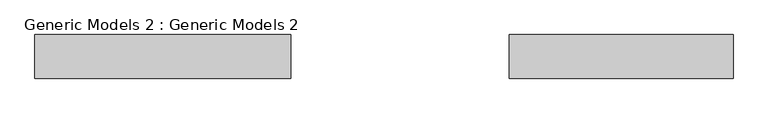
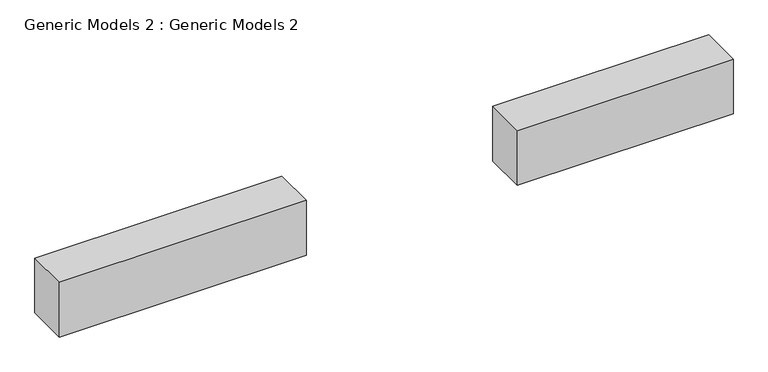
"""IFC4 building model written with IfcOpenShell, lengths in millimetres: proxy geometry, Generic Models 2 : Generic Models 2."""

from ifc_helpers import new_model, si_unit, frame, origin, place, context, project, spatial, polyline, outline, extrude, source, transform, mapped, element, save


def generic_models_2_generic_models_2_263b720d(model_context):
    return source(origin(), model_context, "Body", "SweptSolid", [
        extrude(outline(polyline([(-3264.7966546, -3075.5600272), (-5051.4108866, -3075.5600272), (-5051.4108866, -2770.7600272), (-3264.7966546, -2770.7600272), (-3264.7966546, -3075.5600272)])), frame((0.0, 0.0, 2476.1418569), z_axis=(0.0, 0.0, 1.0), x_axis=(1.0, 0.0, 0.0)), (0.0, 0.0, 1.0), 419.4581431),
        extrude(outline(polyline([(-174.6108866, -3075.5600272), (-1736.7108866, -3075.5600272), (-1736.7108866, -2770.7600272), (-174.6108866, -2770.7600272), (-174.6108866, -3075.5600272)])), frame((0.0, 0.0, 2476.1418569), z_axis=(0.0, 0.0, 1.0), x_axis=(1.0, 0.0, 0.0)), (0.0, 0.0, 1.0), 419.4581431),
    ])


if __name__ == "__main__":
    model = new_model("IFC4")
    model_context = context("Model", 3, world=origin())
    ifc_project = project(units=[si_unit("LENGTHUNIT", "METRE", prefix="MILLI")], contexts=[model_context])
    site = spatial("IfcSite", under=ifc_project)
    building = spatial("IfcBuilding", under=site)
    placement = place(None, origin())
    generic_models_2_generic_models_2_shape = generic_models_2_generic_models_2_263b720d(model_context)
    element("IfcBuildingElementProxy", 1, Name="Generic Models 2 : Generic Models 2", ObjectType="Generic Models 2 : Generic Models 2", at=placement, inside=building, context=model_context, shape_type="MappedRepresentation", body=[
        mapped(generic_models_2_generic_models_2_shape, transform((0.0, 0.0, 0.0), x_axis=(1.0, 0.0, 0.0), y_axis=(0.0, 1.0, 0.0), z_axis=(0.0, 0.0, 1.0))),
    ])
    save(model, "model.ifc")
